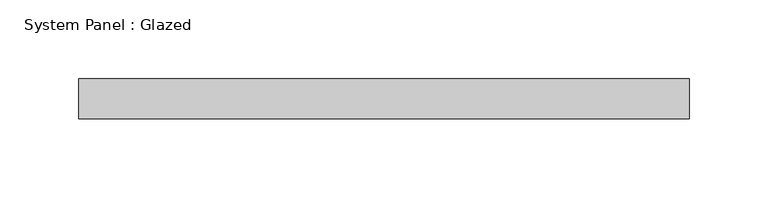
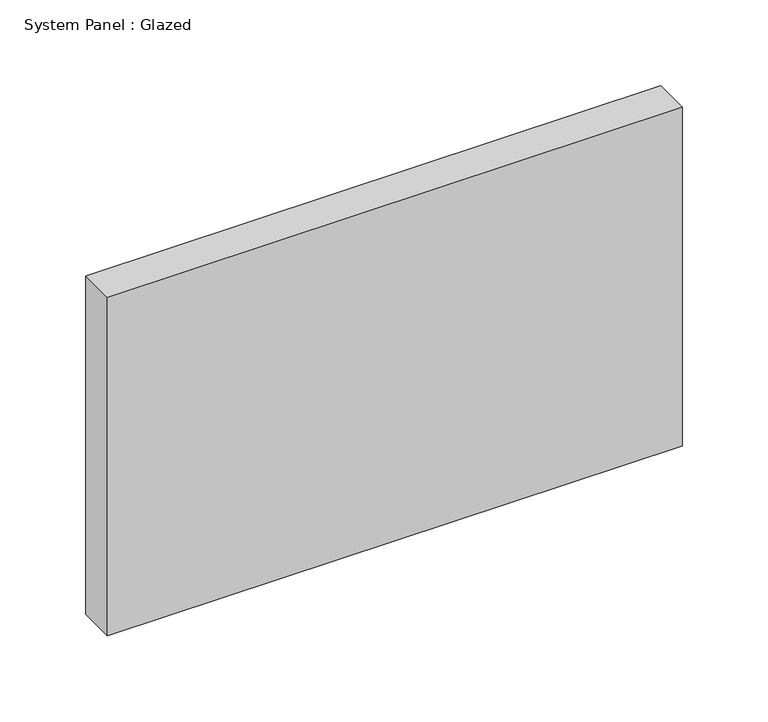
"""IFC4 building model written with IfcOpenShell, lengths in millimetres: plate geometry, System Panel : Glazed."""

from ifc_helpers import new_model, si_unit, origin, origin_with_axes, place, context, project, spatial, polyline, outline, extrude, source, transform, mapped, element, save


def system_panel_glazed_e947191b(model_context):
    return source(origin(), model_context, "Body", "SweptSolid", [
        extrude(outline(polyline([(193.675, 19.05), (-193.675, 19.05), (-193.675, 44.45), (193.675, 44.45), (193.675, 19.05)])), origin_with_axes(), (0.0, 0.0, 1.0), 241.3),
    ])


if __name__ == "__main__":
    model = new_model("IFC4")
    model_context = context("Model", 3, world=origin())
    ifc_project = project(units=[si_unit("LENGTHUNIT", "METRE", prefix="MILLI")], contexts=[model_context])
    site = spatial("IfcSite", under=ifc_project)
    building = spatial("IfcBuilding", under=site)
    placement = place(None, origin())
    system_panel_glazed_shape = system_panel_glazed_e947191b(model_context)
    element("IfcPlate", 1, ObjectType="System Panel : Glazed", at=placement, inside=building, context=model_context, shape_type="MappedRepresentation", body=[
        mapped(system_panel_glazed_shape, transform((0.0, 0.0, 0.0), x_axis=(1.0, 0.0, 0.0), y_axis=(0.0, 1.0, 0.0), z_axis=(0.0, 0.0, 1.0))),
    ])
    save(model, "model.ifc")

# Revit data of these elements
# Type "System Panel : Glazed"
#   Construction Type Id = "GSP4R"
#   Analytic Construction = "1/8 in Pilkington single glazing"
#   Visual Light Transmittance = 0.9
#   Solar Heat Gain Coefficient = 0.86
#   Heat Transfer Coefficient (U) = 1.18115 BTU/(h·ft²·°F)
#   Define Thermal Properties by = 1
# Element 1 (IfcPlate, "System Panel : Glazed")
#   Materials on its faces: "Glass"
# Materials
#   "Glass": class "Glass", colour RGB 0 128 192, transparency 0.75, Description = "Soda Lime Glass", Cost = 0
